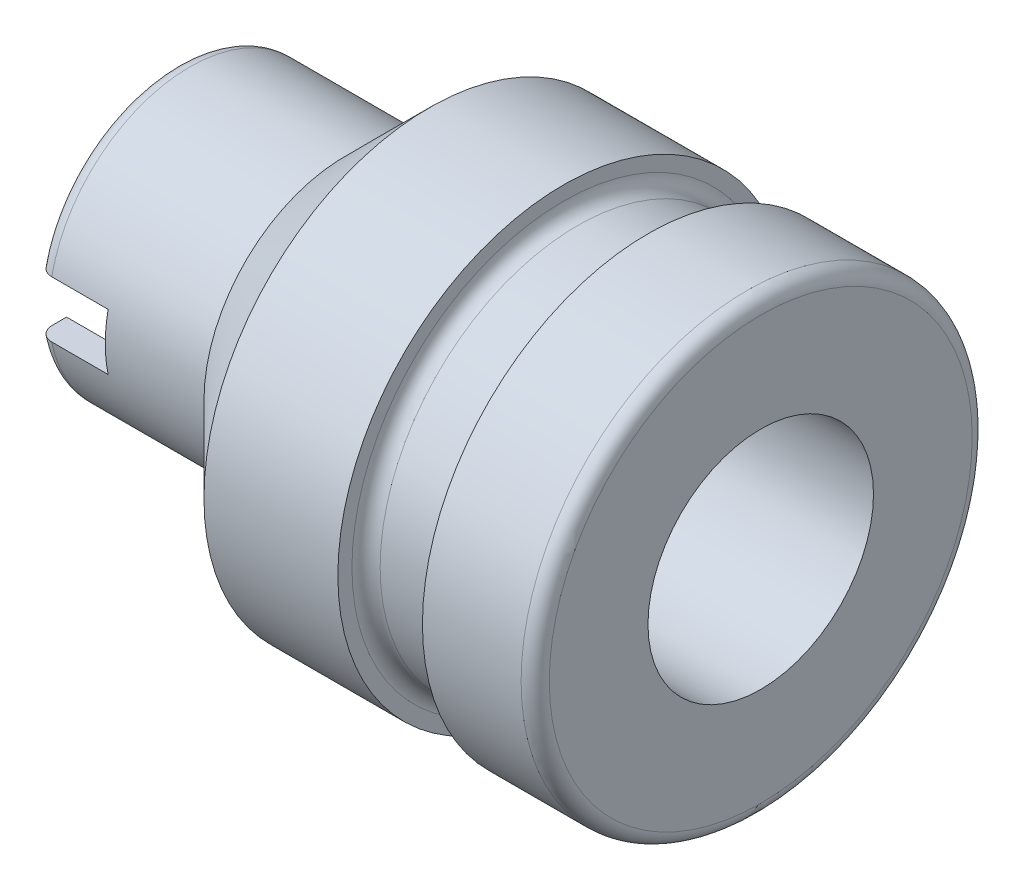
ISO-10303-21;
HEADER;
FILE_DESCRIPTION(('STEP AP214'),'2;1');
FILE_NAME('part.step','',(''),(''),'','','');
FILE_SCHEMA(('AUTOMOTIVE_DESIGN { 1 0 10303 214 1 1 1 1 }'));
ENDSEC;
DATA;
#1=APPLICATION_CONTEXT('core data for automotive mechanical design processes');
#2=APPLICATION_PROTOCOL_DEFINITION('international standard','automotive_design',2000,#1);
#3=PRODUCT_CONTEXT('',#1,'mechanical');
#4=PRODUCT('Part','Part','',(#3));
#5=PRODUCT_RELATED_PRODUCT_CATEGORY('part','',(#4));
#6=PRODUCT_DEFINITION_FORMATION('','',#4);
#7=PRODUCT_DEFINITION_CONTEXT('part definition',#1,'design');
#8=PRODUCT_DEFINITION('design','',#6,#7);
#9=PRODUCT_DEFINITION_SHAPE('','',#8);
#10=(LENGTH_UNIT() NAMED_UNIT(*) SI_UNIT(.MILLI.,.METRE.));
#11=(NAMED_UNIT(*) PLANE_ANGLE_UNIT() SI_UNIT($,.RADIAN.));
#12=(NAMED_UNIT(*) SI_UNIT($,.STERADIAN.) SOLID_ANGLE_UNIT());
#13=UNCERTAINTY_MEASURE_WITH_UNIT(LENGTH_MEASURE(1.E-05),#10,'distance_accuracy_value','');
#14=(GEOMETRIC_REPRESENTATION_CONTEXT(3) GLOBAL_UNCERTAINTY_ASSIGNED_CONTEXT((#13)) GLOBAL_UNIT_ASSIGNED_CONTEXT((#10,
#11,#12)) REPRESENTATION_CONTEXT('',''));
#15=CARTESIAN_POINT('',(0.,0.,0.));
#16=DIRECTION('',(0.,0.,1.));
#17=DIRECTION('',(1.,0.,0.));
#18=AXIS2_PLACEMENT_3D('',#15,#16,#17);
#19=CARTESIAN_POINT('',(0.,0.,0.));
#20=DIRECTION('',(-1.,0.,0.));
#21=DIRECTION('',(0.,0.,1.));
#22=AXIS2_PLACEMENT_3D('',#19,#20,#21);
#23=PLANE('',#22);
#24=DIRECTION('',(0.,0.,1.));
#25=VECTOR('',#24,1.);
#26=CARTESIAN_POINT('',(0.,10.,-16.));
#27=LINE('',#26,#25);
#28=CARTESIAN_POINT('',(0.,10.,7.74596669241483));
#29=VERTEX_POINT('',#28);
#30=CARTESIAN_POINT('',(0.,10.,8.7749643873921));
#31=VERTEX_POINT('',#30);
#32=EDGE_CURVE('E194',#29,#31,#27,.T.);
#33=ORIENTED_EDGE('',*,*,#32,.T.);
#34=CARTESIAN_POINT('',(0.,8.,0.));
#35=DIRECTION('',(-1.,0.,0.));
#36=DIRECTION('',(0.,0.,1.));
#37=AXIS2_PLACEMENT_3D('',#34,#35,#36);
#38=CIRCLE('',#37,8.99999999999998);
#39=CARTESIAN_POINT('',(0.,10.,-8.77496438739202));
#40=VERTEX_POINT('',#39);
#41=EDGE_CURVE('E220',#31,#40,#38,.T.);
#42=ORIENTED_EDGE('',*,*,#41,.T.);
#43=CARTESIAN_POINT('',(0.,10.,-7.74596669241483));
#44=VERTEX_POINT('',#43);
#45=EDGE_CURVE('E193',#40,#44,#27,.T.);
#46=ORIENTED_EDGE('',*,*,#45,.T.);
#47=CARTESIAN_POINT('',(0.,8.,0.));
#48=DIRECTION('',(-1.,0.,0.));
#49=DIRECTION('',(0.,0.,1.));
#50=AXIS2_PLACEMENT_3D('',#47,#48,#49);
#51=CIRCLE('',#50,8.);
#52=EDGE_CURVE('E223',#29,#44,#51,.T.);
#53=ORIENTED_EDGE('',*,*,#52,.F.);
#54=EDGE_LOOP('',(#33,#42,#46,#53));
#55=FACE_BOUND('',#54,.T.);
#56=ADVANCED_FACE('F44',(#55),#23,.T.);
#57=CARTESIAN_POINT('',(1.,8.,0.));
#58=DIRECTION('',(-1.,0.,0.));
#59=DIRECTION('',(0.,0.,1.));
#60=AXIS2_PLACEMENT_3D('',#57,#58,#59);
#61=TOROIDAL_SURFACE('',#60,8.99999999999998,1.);
#62=CARTESIAN_POINT('',(0.511306825927035,10.,-9.6677495790696));
#63=CARTESIAN_POINT('',(0.559308281722965,10.,-9.69520351096408));
#64=CARTESIAN_POINT('',(0.609639032154946,10.,-9.71865802064844));
#65=CARTESIAN_POINT('',(0.713558242155809,10.,-9.75681559968103));
#66=CARTESIAN_POINT('',(0.767149945956613,10.,-9.77150979140529));
#67=CARTESIAN_POINT('',(0.876043559476013,10.,-9.79166035519747));
#68=CARTESIAN_POINT('',(0.931345300899028,10.,-9.79711763340043));
#69=CARTESIAN_POINT('',(1.04206355524924,10.,-9.79861988345027));
#70=CARTESIAN_POINT('',(1.09748004028236,10.,-9.7946669235582));
#71=CARTESIAN_POINT('',(1.20660988208594,10.,-9.77751812422735));
#72=CARTESIAN_POINT('',(1.26032970143437,10.,-9.76436334861136));
#73=CARTESIAN_POINT('',(1.36481599217086,10.,-9.72926499149187));
#74=CARTESIAN_POINT('',(1.41558235227585,10.,-9.70732107906873));
#75=CARTESIAN_POINT('',(1.51301248392595,10.,-9.65518458376579));
#76=CARTESIAN_POINT('',(1.5596543139653,10.,-9.62495102864483));
#77=CARTESIAN_POINT('',(1.647298612418,10.,-9.5571938737038));
#78=CARTESIAN_POINT('',(1.68830072482487,10.,-9.51966981403191));
#79=CARTESIAN_POINT('',(1.76419505830093,10.,-9.43779402545148));
#80=CARTESIAN_POINT('',(1.79898312438137,10.,-9.39334578929934));
#81=CARTESIAN_POINT('',(1.86078526900064,10.,-9.29934095322765));
#82=CARTESIAN_POINT('',(1.88779856031153,10.,-9.24978383670244));
#83=CARTESIAN_POINT('',(1.93389245120233,10.,-9.14584851749056));
#84=CARTESIAN_POINT('',(1.95279295699506,10.,-9.09139044671483));
#85=CARTESIAN_POINT('',(1.98138125003641,10.,-8.98010780940885));
#86=CARTESIAN_POINT('',(1.99106799193015,10.,-8.9232829751188));
#87=CARTESIAN_POINT('',(2.00112427890071,10.,-8.80768146328481));
#88=CARTESIAN_POINT('',(2.00130601462751,10.,-8.74888840256496));
#89=CARTESIAN_POINT('',(1.9919017520578,10.,-8.63208632529093));
#90=CARTESIAN_POINT('',(1.98231495867919,10.,-8.57407737294647));
#91=CARTESIAN_POINT('',(1.95348329284294,10.,-8.45989655601053));
#92=CARTESIAN_POINT('',(1.93414395709675,10.,-8.40374849719579));
#93=CARTESIAN_POINT('',(1.8862524674463,10.,-8.29552412270311));
#94=CARTESIAN_POINT('',(1.85770032889892,10.,-8.24344780023816));
#95=CARTESIAN_POINT('',(1.79234125019335,10.,-8.14526750270985));
#96=CARTESIAN_POINT('',(1.75559179207176,10.,-8.09912530594951));
#97=CARTESIAN_POINT('',(1.67469797107571,10.,-8.01385024714823));
#98=CARTESIAN_POINT('',(1.63055451541159,10.,-7.97471652641611));
#99=CARTESIAN_POINT('',(1.53721783151604,10.,-7.90558984461912));
#100=CARTESIAN_POINT('',(1.48816814766731,10.,-7.87540317887255));
#101=CARTESIAN_POINT('',(1.38557805500345,10.,-7.82398855871157));
#102=CARTESIAN_POINT('',(1.33203850957662,10.,-7.80275888660533));
#103=CARTESIAN_POINT('',(1.22370997690863,10.,-7.77050867101741));
#104=CARTESIAN_POINT('',(1.16900603361279,10.,-7.75920221435131));
#105=CARTESIAN_POINT('',(1.05847182518937,10.,-7.74613510599163));
#106=CARTESIAN_POINT('',(1.00264171380159,10.,-7.74437316005553));
#107=CARTESIAN_POINT('',(0.892582708877808,10.,-7.75039635440434));
#108=CARTESIAN_POINT('',(0.838343678634541,10.,-7.75799839748392));
#109=CARTESIAN_POINT('',(0.731908480522575,10.,-7.78217880416063));
#110=CARTESIAN_POINT('',(0.679712293696711,10.,-7.79875708443894));
#111=CARTESIAN_POINT('',(0.578658081208827,10.,-7.84039550056985));
#112=CARTESIAN_POINT('',(0.529809656562754,10.,-7.86547889710702));
#113=CARTESIAN_POINT('',(0.43689225974382,10.,-7.92331749551591));
#114=CARTESIAN_POINT('',(0.392823751135206,10.,-7.95607344051264));
#115=CARTESIAN_POINT('',(0.309637769043108,10.,-8.02908979521609));
#116=CARTESIAN_POINT('',(0.270654071066901,10.,-8.06950253140811));
#117=CARTESIAN_POINT('',(0.199789029681809,10.,-8.15613564920241));
#118=CARTESIAN_POINT('',(0.167908744225208,10.,-8.20235689429834));
#119=CARTESIAN_POINT('',(0.11118055267698,10.,-8.3007507838291));
#120=CARTESIAN_POINT('',(0.0865663966446748,10.,-8.35305824482765));
#121=CARTESIAN_POINT('',(0.0462562889607229,10.,-8.46100433264482));
#122=CARTESIAN_POINT('',(0.0305614855014643,10.,-8.51664338732247));
#123=CARTESIAN_POINT('',(0.00823822667101209,10.,-8.63095929611147));
#124=CARTESIAN_POINT('',(0.00181209474607875,10.,-8.68967575315516));
#125=CARTESIAN_POINT('',(-0.001147154551948,10.,-8.80735800605802));
#126=CARTESIAN_POINT('',(0.00231987019037505,10.,-8.86632380548684));
#127=CARTESIAN_POINT('',(0.0191336971782254,10.,-8.98312733812228));
#128=CARTESIAN_POINT('',(0.0325285171266589,10.,-9.04095818168231));
#129=CARTESIAN_POINT('',(0.068952109280189,10.,-9.15352293406955));
#130=CARTESIAN_POINT('',(0.091982863025496,10.,-9.2082562032797));
#131=CARTESIAN_POINT('',(0.146792032565864,10.,-9.31239064575795));
#132=CARTESIAN_POINT('',(0.178472817770748,10.,-9.36184323216501));
#133=CARTESIAN_POINT('',(0.249831530740876,10.,-9.45453280413945));
#134=CARTESIAN_POINT('',(0.289498801103796,10.,-9.4977779427507));
#135=CARTESIAN_POINT('',(0.35984513733962,10.,-9.56220360357953));
#136=CARTESIAN_POINT('',(0.388477869102997,10.,-9.5856561085426));
#137=CARTESIAN_POINT('',(0.448162302179852,10.,-9.62925148252653));
#138=CARTESIAN_POINT('',(0.479213966106138,10.,-9.64939440268562));
#139=CARTESIAN_POINT('',(0.511306825927035,10.,-9.6677495790696));
#140=B_SPLINE_CURVE_WITH_KNOTS('',3,(#62,#63,#64,#65,#66,#67,#68,#69,#70,#71,#72,#73,#74,#75,
#76,#77,#78,#79,#80,#81,#82,#83,#84,#85,#86,#87,#88,#89,#90,#91,#92,#93,#94,#95,#96,#97,#98,#99,
#100,#101,#102,#103,#104,#105,#106,#107,#108,#109,#110,#111,#112,#113,#114,#115,#116,#117,#118,
#119,#120,#121,#122,#123,#124,#125,#126,#127,#128,#129,#130,#131,#132,#133,#134,#135,#136,#137,
#138,#139),.UNSPECIFIED.,.T.,.F.,(4,2,2,2,2,2,2,2,2,2,2,2,2,2,2,2,2,2,2,2,2,2,2,2,2,2,2,2,2,2,2,
2,2,2,2,2,2,2,4),(0.,0.165760656846688,0.331689009703769,0.497601084156693,0.66347669642919,
0.828616759413993,0.993763040669096,1.15974076125184,1.32572895435387,1.49428098685655,
1.66285007994709,1.8349887499326,2.0071469477183,2.18270555882353,2.35827846017236,
2.53558560043269,2.71289244514009,2.88899300563287,3.06507197518268,3.23700082338466,
3.40889668561266,3.57565978746695,3.74240027555845,3.90593155970491,4.06946132595477,
4.23344198705861,4.39743853708843,4.56512660663086,4.7328396342577,4.9054729168679,
5.0781284176095,5.25449852909511,5.43087117415406,5.60810249270579,5.78537027515778,
5.96071456378588,6.13582640039848,6.24665253354264,6.35747695408974),.UNSPECIFIED.);
#141=CARTESIAN_POINT('',(1.,10.,-9.79795897113269));
#142=VERTEX_POINT('',#141);
#143=EDGE_CURVE('E156',#40,#142,#140,.T.);
#144=ORIENTED_EDGE('',*,*,#143,.F.);
#145=ORIENTED_EDGE('',*,*,#41,.F.);
#146=CARTESIAN_POINT('',(0.530086633266854,10.,7.8670423739127));
#147=CARTESIAN_POINT('',(0.578141397714327,10.,7.84064914283677));
#148=CARTESIAN_POINT('',(0.628419871150143,10.,7.81823476131326));
#149=CARTESIAN_POINT('',(0.732054975608554,10.,7.78212334392136));
#150=CARTESIAN_POINT('',(0.785414272238746,10.,7.76843398426953));
#151=CARTESIAN_POINT('',(0.893694754150047,10.,7.7502583049771));
#152=CARTESIAN_POINT('',(0.94861621718662,10.,7.74577363244534));
#153=CARTESIAN_POINT('',(1.05841316345902,10.,7.74617251060403));
#154=CARTESIAN_POINT('',(1.1132886538094,10.,7.75105414228967));
#155=CARTESIAN_POINT('',(1.22101648805253,10.,7.76993821482575));
#156=CARTESIAN_POINT('',(1.27388095611584,10.,7.78387168868395));
#157=CARTESIAN_POINT('',(1.37655874242189,10.,7.82032521094701));
#158=CARTESIAN_POINT('',(1.42637187394239,10.,7.8428457842193));
#159=CARTESIAN_POINT('',(1.52213173794623,10.,7.89603321356496));
#160=CARTESIAN_POINT('',(1.56803166365623,10.,7.92678424161405));
#161=CARTESIAN_POINT('',(1.65419034084942,10.,7.9953682486375));
#162=CARTESIAN_POINT('',(1.69444840750263,10.,8.03320208605009));
#163=CARTESIAN_POINT('',(1.76933370530235,10.,8.11594516892443));
#164=CARTESIAN_POINT('',(1.8037821363678,10.,8.16101619860671));
#165=CARTESIAN_POINT('',(1.8648692450916,10.,8.25617083413549));
#166=CARTESIAN_POINT('',(1.89150677818158,10.,8.30625517316537));
#167=CARTESIAN_POINT('',(1.93697477776608,10.,8.41152787043869));
#168=CARTESIAN_POINT('',(1.9555650521892,10.,8.46682005042279));
#169=CARTESIAN_POINT('',(1.98336758010917,10.,8.57971552998892));
#170=CARTESIAN_POINT('',(1.99257883459075,10.,8.63731907508913));
#171=CARTESIAN_POINT('',(2.00145172674255,10.,8.75420255934511));
#172=CARTESIAN_POINT('',(2.00095588058722,10.,8.81349453153748));
#173=CARTESIAN_POINT('',(1.99000786091946,10.,8.93115517583231));
#174=CARTESIAN_POINT('',(1.97955550413699,10.,8.98952383091912));
#175=CARTESIAN_POINT('',(1.94894306490324,10.,9.10358714712749));
#176=CARTESIAN_POINT('',(1.92879463966272,10.,9.15928493113948));
#177=CARTESIAN_POINT('',(1.87928764906859,10.,9.26642836714244));
#178=CARTESIAN_POINT('',(1.84992973339864,10.,9.31787431875565));
#179=CARTESIAN_POINT('',(1.78330190216955,10.,9.41417425155647));
#180=CARTESIAN_POINT('',(1.74616272288383,10.,9.45911864051572));
#181=CARTESIAN_POINT('',(1.66471340194489,10.,9.54195979436287));
#182=CARTESIAN_POINT('',(1.62040412592035,10.,9.57985740880559));
#183=CARTESIAN_POINT('',(1.52691131817347,10.,9.64664863756471));
#184=CARTESIAN_POINT('',(1.47785526132285,10.,9.67572069984084));
#185=CARTESIAN_POINT('',(1.37548685852437,10.,9.72502935448071));
#186=CARTESIAN_POINT('',(1.32217501009044,10.,9.74526697783106));
#187=CARTESIAN_POINT('',(1.21391011756111,10.,9.77595055141352));
#188=CARTESIAN_POINT('',(1.15900809567203,10.,9.78657669499911));
#189=CARTESIAN_POINT('',(1.04819822807474,10.,9.79835661860274));
#190=CARTESIAN_POINT('',(0.992290455428851,10.,9.79951108392428));
#191=CARTESIAN_POINT('',(0.881654127451369,10.,9.79234847781777));
#192=CARTESIAN_POINT('',(0.826919366226506,10.,9.78412675678912));
#193=CARTESIAN_POINT('',(0.719604454653113,10.,9.75862572790174));
#194=CARTESIAN_POINT('',(0.667024283713556,10.,9.74134650662567));
#195=CARTESIAN_POINT('',(0.565390440348432,10.,9.69822660717811));
#196=CARTESIAN_POINT('',(0.516343373928049,10.,9.67237037327907));
#197=CARTESIAN_POINT('',(0.423212995336157,10.,9.61289096461068));
#198=CARTESIAN_POINT('',(0.379129927662664,10.,9.57926740751637));
#199=CARTESIAN_POINT('',(0.296548199057912,10.,9.50476302258947));
#200=CARTESIAN_POINT('',(0.258129456500358,10.,9.46379365494053));
#201=CARTESIAN_POINT('',(0.188551954038964,10.,9.37609769672073));
#202=CARTESIAN_POINT('',(0.157393896303961,10.,9.32937054999207));
#203=CARTESIAN_POINT('',(0.102544847496919,10.,9.23047974526343));
#204=CARTESIAN_POINT('',(0.0790177674306911,10.,9.17822518894706));
#205=CARTESIAN_POINT('',(0.0408664514457591,10.,9.07056209938669));
#206=CARTESIAN_POINT('',(0.026243238739463,10.,9.01515320445294));
#207=CARTESIAN_POINT('',(0.00601242351154127,10.,8.90151246286388));
#208=CARTESIAN_POINT('',(0.000600274872774322,10.,8.8432457862255));
#209=CARTESIAN_POINT('',(-0.000505796595671923,10.,8.72662072581589));
#210=CARTESIAN_POINT('',(0.00380084075076319,10.,8.66826233695224));
#211=CARTESIAN_POINT('',(0.0221249794561776,10.,8.55229379625042));
#212=CARTESIAN_POINT('',(0.0362704171598719,10.,8.49470380971241));
#213=CARTESIAN_POINT('',(0.0740488816321859,10.,8.38270291383713));
#214=CARTESIAN_POINT('',(0.0976844683595091,10.,8.3282928668258));
#215=CARTESIAN_POINT('',(0.153795894139131,10.,8.22434078489802));
#216=CARTESIAN_POINT('',(0.186259004324004,10.,8.17479187937067));
#217=CARTESIAN_POINT('',(0.259176927714039,10.,8.08203325396201));
#218=CARTESIAN_POINT('',(0.299621370850104,10.,8.03881543379349));
#219=CARTESIAN_POINT('',(0.371936794602742,10.,7.9739318252388));
#220=CARTESIAN_POINT('',(0.401830277842509,10.,7.95002752103271));
#221=CARTESIAN_POINT('',(0.464151019596761,10.,7.90578479045156));
#222=CARTESIAN_POINT('',(0.496578217983059,10.,7.88544627949296));
#223=CARTESIAN_POINT('',(0.530086633266854,10.,7.8670423739127));
#224=B_SPLINE_CURVE_WITH_KNOTS('',3,(#146,#147,#148,#149,#150,#151,#152,#153,#154,#155,#156,
#157,#158,#159,#160,#161,#162,#163,#164,#165,#166,#167,#168,#169,#170,#171,#172,#173,#174,#175,
#176,#177,#178,#179,#180,#181,#182,#183,#184,#185,#186,#187,#188,#189,#190,#191,#192,#193,#194,
#195,#196,#197,#198,#199,#200,#201,#202,#203,#204,#205,#206,#207,#208,#209,#210,#211,#212,#213,
#214,#215,#216,#217,#218,#219,#220,#221,#222,#223),.UNSPECIFIED.,.T.,.F.,(4,2,2,2,2,2,2,2,2,2,2,
2,2,2,2,2,2,2,2,2,2,2,2,2,2,2,2,2,2,2,2,2,2,2,2,2,2,2,4),(0.,0.164341324993714,
0.328827037538444,0.493342180986613,0.657823621532061,0.821066328878155,0.984319015672965,
1.14930967077576,1.31432033574771,1.48373163535811,1.6531677472279,1.827361011495,
2.00157282818377,2.17861329102043,2.35565701271359,2.53248841130041,2.70930733811718,
2.88336459438589,3.05740085279306,3.22763906699898,3.3978574089444,3.56481409859054,
3.73175870832779,3.89702061163649,4.06228093519885,4.22784263754271,4.39341249093985,
4.56113157984433,4.72886688185976,4.8999974046941,5.07114758975335,5.24588619185384,
5.42063486588012,5.59769938739947,5.77481170402832,5.95166997514037,6.12829995124597,
6.24289728777437,6.35749190559209),.UNSPECIFIED.);
#225=CARTESIAN_POINT('',(1.,10.,9.79795897113269));
#226=VERTEX_POINT('',#225);
#227=EDGE_CURVE('E150',#226,#31,#224,.T.);
#228=ORIENTED_EDGE('',*,*,#227,.F.);
#229=CARTESIAN_POINT('',(1.,8.,0.));
#230=DIRECTION('',(-1.,0.,0.));
#231=DIRECTION('',(0.,0.,1.));
#232=AXIS2_PLACEMENT_3D('',#229,#230,#231);
#233=CIRCLE('',#232,9.99999999999998);
#234=EDGE_CURVE('E217',#226,#142,#233,.T.);
#235=ORIENTED_EDGE('',*,*,#234,.T.);
#236=EDGE_LOOP('',(#144,#145,#228,#235));
#237=FACE_BOUND('',#236,.T.);
#238=ADVANCED_FACE('F248',(#237),#61,.T.);
#239=CARTESIAN_POINT('',(-18.7543710445799,8.,0.));
#240=DIRECTION('',(-1.,0.,0.));
#241=DIRECTION('',(0.,0.,1.));
#242=AXIS2_PLACEMENT_3D('',#239,#240,#241);
#243=CYLINDRICAL_SURFACE('',#242,8.);
#244=DIRECTION('',(-1.,0.,0.));
#245=VECTOR('',#244,1.);
#246=CARTESIAN_POINT('',(-18.7543710445799,10.,7.74596669241483));
#247=LINE('',#246,#245);
#248=CARTESIAN_POINT('',(5.,10.,7.74596669241483));
#249=VERTEX_POINT('',#248);
#250=EDGE_CURVE('E239',#29,#249,#247,.F.);
#251=ORIENTED_EDGE('',*,*,#250,.F.);
#252=ORIENTED_EDGE('',*,*,#52,.T.);
#253=DIRECTION('',(-1.,0.,0.));
#254=VECTOR('',#253,1.);
#255=CARTESIAN_POINT('',(-18.7543710445799,10.,-7.74596669241483));
#256=LINE('',#255,#254);
#257=CARTESIAN_POINT('',(5.,10.,-7.74596669241483));
#258=VERTEX_POINT('',#257);
#259=EDGE_CURVE('E145',#258,#44,#256,.T.);
#260=ORIENTED_EDGE('',*,*,#259,.F.);
#261=CARTESIAN_POINT('',(5.,8.,0.));
#262=DIRECTION('',(1.,0.,0.));
#263=DIRECTION('',(0.,0.,-1.));
#264=AXIS2_PLACEMENT_3D('',#261,#262,#263);
#265=CIRCLE('',#264,8.);
#266=CARTESIAN_POINT('',(5.,6.,-7.74596669241483));
#267=VERTEX_POINT('',#266);
#268=EDGE_CURVE('E135',#267,#258,#265,.T.);
#269=ORIENTED_EDGE('',*,*,#268,.F.);
#270=DIRECTION('',(-1.,0.,0.));
#271=VECTOR('',#270,1.);
#272=CARTESIAN_POINT('',(-18.7543710445799,6.,-7.74596669241483));
#273=LINE('',#272,#271);
#274=CARTESIAN_POINT('',(0.,6.,-7.74596669241483));
#275=VERTEX_POINT('',#274);
#276=EDGE_CURVE('E116',#275,#267,#273,.F.);
#277=ORIENTED_EDGE('',*,*,#276,.F.);
#278=CARTESIAN_POINT('',(0.,6.,7.74596669241483));
#279=VERTEX_POINT('',#278);
#280=EDGE_CURVE('E219',#275,#279,#51,.T.);
#281=ORIENTED_EDGE('',*,*,#280,.T.);
#282=DIRECTION('',(-1.,0.,0.));
#283=VECTOR('',#282,1.);
#284=CARTESIAN_POINT('',(-18.7543710445799,6.,7.74596669241483));
#285=LINE('',#284,#283);
#286=CARTESIAN_POINT('',(5.,6.,7.74596669241483));
#287=VERTEX_POINT('',#286);
#288=EDGE_CURVE('E130',#287,#279,#285,.T.);
#289=ORIENTED_EDGE('',*,*,#288,.F.);
#290=EDGE_CURVE('E144',#249,#287,#265,.T.);
#291=ORIENTED_EDGE('',*,*,#290,.F.);
#292=EDGE_LOOP('',(#251,#252,#260,#269,#277,#281,#289,#291));
#293=FACE_BOUND('',#292,.T.);
#294=CARTESIAN_POINT('',(41.5,8.,0.));
#295=DIRECTION('',(-1.,0.,0.));
#296=DIRECTION('',(0.,0.,1.));
#297=AXIS2_PLACEMENT_3D('',#294,#295,#296);
#298=CIRCLE('',#297,7.99999999999999);
#299=CARTESIAN_POINT('',(41.5,8.,7.99999999999999));
#300=VERTEX_POINT('',#299);
#301=EDGE_CURVE('E246',#300,#300,#298,.T.);
#302=ORIENTED_EDGE('',*,*,#301,.F.);
#303=EDGE_LOOP('',(#302));
#304=FACE_BOUND('',#303,.T.);
#305=ADVANCED_FACE('F50',(#293,#304),#243,.F.);
#306=DIRECTION('',(0.,0.,1.));
#307=VECTOR('',#306,1.);
#308=CARTESIAN_POINT('',(0.,6.,-16.));
#309=LINE('',#308,#307);
#310=CARTESIAN_POINT('',(0.,6.,-8.77496438739146));
#311=VERTEX_POINT('',#310);
#312=EDGE_CURVE('E125',#311,#275,#309,.T.);
#313=ORIENTED_EDGE('',*,*,#312,.F.);
#314=CARTESIAN_POINT('',(0.,6.,8.77496438739227));
#315=VERTEX_POINT('',#314);
#316=EDGE_CURVE('E213',#311,#315,#38,.T.);
#317=ORIENTED_EDGE('',*,*,#316,.T.);
#318=EDGE_CURVE('E204',#279,#315,#309,.T.);
#319=ORIENTED_EDGE('',*,*,#318,.F.);
#320=ORIENTED_EDGE('',*,*,#280,.F.);
#321=EDGE_LOOP('',(#313,#317,#319,#320));
#322=FACE_BOUND('',#321,.T.);
#323=ADVANCED_FACE('F216',(#322),#23,.T.);
#324=CARTESIAN_POINT('',(0.511306825927035,6.,-9.6677495790696));
#325=CARTESIAN_POINT('',(0.462127792878772,6.,-9.63961614014446));
#326=CARTESIAN_POINT('',(0.415321432721198,6.,-9.60724164376228));
#327=CARTESIAN_POINT('',(0.327807674940792,6.,-9.53502366722364));
#328=CARTESIAN_POINT('',(0.287109053947641,6.,-9.49516962067705));
#329=CARTESIAN_POINT('',(0.212996868443189,6.,-9.40927866329832));
#330=CARTESIAN_POINT('',(0.179573316452268,6.,-9.36325037090132));
#331=CARTESIAN_POINT('',(0.120796696181657,6.,-9.26632548183998));
#332=CARTESIAN_POINT('',(0.0954416705950956,6.,-9.21543006976995));
#333=CARTESIAN_POINT('',(0.05305026963304,6.,-9.10933538170457));
#334=CARTESIAN_POINT('',(0.0361541675774601,6.,-9.05408007300957));
#335=CARTESIAN_POINT('',(0.0116835589855953,6.,-8.94153981509048));
#336=CARTESIAN_POINT('',(0.00411048112851551,6.,-8.88425455617609));
#337=CARTESIAN_POINT('',(-0.00161449656823779,6.,-8.76811550635739));
#338=CARTESIAN_POINT('',(0.000416367341279644,6.,-8.7092526583363));
#339=CARTESIAN_POINT('',(0.0142429607025673,6.,-8.59268248788178));
#340=CARTESIAN_POINT('',(0.0260394125136054,6.,-8.53497525125219));
#341=CARTESIAN_POINT('',(0.0592295532006887,6.,-8.42186663703923));
#342=CARTESIAN_POINT('',(0.0807017165191936,6.,-8.36648824519507));
#343=CARTESIAN_POINT('',(0.132717456638743,6.,-8.26016420202981));
#344=CARTESIAN_POINT('',(0.163260879747507,6.,-8.20921847562597));
#345=CARTESIAN_POINT('',(0.232319712500392,6.,-8.11373419885014));
#346=CARTESIAN_POINT('',(0.270761984519968,6.,-8.06914281018449));
#347=CARTESIAN_POINT('',(0.35475961241516,6.,-7.9872504066813));
#348=CARTESIAN_POINT('',(0.400314015263732,6.,-7.94994841656858));
#349=CARTESIAN_POINT('',(0.49603998492741,6.,-7.88472033956897));
#350=CARTESIAN_POINT('',(0.546067638456784,6.,-7.85658315502762));
#351=CARTESIAN_POINT('',(0.650242201905039,6.,-7.80940325123956));
#352=CARTESIAN_POINT('',(0.704388317457524,6.,-7.79035878332612));
#353=CARTESIAN_POINT('',(0.81354111836697,6.,-7.76246756444927));
#354=CARTESIAN_POINT('',(0.868475209312162,6.,-7.75333635979499));
#355=CARTESIAN_POINT('',(0.97909332477837,6.,-7.74460503194061));
#356=CARTESIAN_POINT('',(1.03477725649985,6.,-7.74500373996807));
#357=CARTESIAN_POINT('',(1.14430583108474,6.,-7.75522657668602));
#358=CARTESIAN_POINT('',(1.19816564263771,6.,-7.76488932614733));
#359=CARTESIAN_POINT('',(1.30351120575465,6.,-7.79307437632797));
#360=CARTESIAN_POINT('',(1.35499694668112,6.,-7.8115967167403));
#361=CARTESIAN_POINT('',(1.45446136037515,6.,-7.85701332402369));
#362=CARTESIAN_POINT('',(1.50241974199559,6.,-7.8839519606661));
#363=CARTESIAN_POINT('',(1.59327424205895,6.,-7.94531836244351));
#364=CARTESIAN_POINT('',(1.63616981903902,6.,-7.97974692750276));
#365=CARTESIAN_POINT('',(1.71679853240975,6.,-8.05598011482791));
#366=CARTESIAN_POINT('',(1.75438273298845,6.,-8.09794219253199));
#367=CARTESIAN_POINT('',(1.82221388314016,6.,-8.18742637731591));
#368=CARTESIAN_POINT('',(1.85245974598291,6.,-8.23494930635633));
#369=CARTESIAN_POINT('',(1.90566745527039,6.,-8.33569399048775));
#370=CARTESIAN_POINT('',(1.92839144874395,6.,-8.38904142784494));
#371=CARTESIAN_POINT('',(1.96476097282934,6.,-8.49874705230807));
#372=CARTESIAN_POINT('',(1.97840540022242,6.,-8.55510560438308));
#373=CARTESIAN_POINT('',(1.99645269595044,6.,-8.67043761172828));
#374=CARTESIAN_POINT('',(2.00066621894879,6.,-8.72944078635048));
#375=CARTESIAN_POINT('',(1.99916261837003,6.,-8.84732326181367));
#376=CARTESIAN_POINT('',(1.9934450951045,6.,-8.9062025575735));
#377=CARTESIAN_POINT('',(1.97215664019017,6.,-9.02233734661196));
#378=CARTESIAN_POINT('',(1.95655657656459,6.,-9.07958751434796));
#379=CARTESIAN_POINT('',(1.9158429235496,6.,-9.19060252497679));
#380=CARTESIAN_POINT('',(1.89072980594297,6.,-9.24436754055462));
#381=CARTESIAN_POINT('',(1.8320123031712,6.,-9.34612633467259));
#382=CARTESIAN_POINT('',(1.79852090549833,6.,-9.39418526504363));
#383=CARTESIAN_POINT('',(1.72378285853897,6.,-9.4838415356261));
#384=CARTESIAN_POINT('',(1.68253707794454,6.,-9.52543959866999));
#385=CARTESIAN_POINT('',(1.59439479967278,6.,-9.60004783335381));
#386=CARTESIAN_POINT('',(1.54763644474854,6.,-9.633221197224));
#387=CARTESIAN_POINT('',(1.44912221996927,6.,-9.69105176991122));
#388=CARTESIAN_POINT('',(1.39736716585799,6.,-9.7157103658215));
#389=CARTESIAN_POINT('',(1.29147850342786,6.,-9.75529780839208));
#390=CARTESIAN_POINT('',(1.23741588921197,6.,-9.77041668772133));
#391=CARTESIAN_POINT('',(1.12749141216315,6.,-9.79123670479128));
#392=CARTESIAN_POINT('',(1.07162923502451,6.,-9.79693618817954));
#393=CARTESIAN_POINT('',(0.960438790024008,6.,-9.798719451814));
#394=CARTESIAN_POINT('',(0.905112274476687,6.,-9.79491913855203));
#395=CARTESIAN_POINT('',(0.795937463990675,6.,-9.7780659133441));
#396=CARTESIAN_POINT('',(0.742087362546607,6.,-9.76502488581324));
#397=CARTESIAN_POINT('',(0.658775688732057,6.,-9.73727365800327));
#398=CARTESIAN_POINT('',(0.62833254518202,6.,-9.7254183911905));
#399=CARTESIAN_POINT('',(0.568765995941057,6.,-9.69876122999197));
#400=CARTESIAN_POINT('',(0.539642573272034,6.,-9.68395937352706));
#401=CARTESIAN_POINT('',(0.511306825927035,6.,-9.6677495790696));
#402=B_SPLINE_CURVE_WITH_KNOTS('',3,(#324,#325,#326,#327,#328,#329,#330,#331,#332,#333,#334,
#335,#336,#337,#338,#339,#340,#341,#342,#343,#344,#345,#346,#347,#348,#349,#350,#351,#352,#353,
#354,#355,#356,#357,#358,#359,#360,#361,#362,#363,#364,#365,#366,#367,#368,#369,#370,#371,#372,
#373,#374,#375,#376,#377,#378,#379,#380,#381,#382,#383,#384,#385,#386,#387,#388,#389,#390,#391,
#392,#393,#394,#395,#396,#397,#398,#399,#400,#401),.UNSPECIFIED.,.T.,.F.,(4,2,2,2,2,2,2,2,2,2,2,
2,2,2,2,2,2,2,2,2,2,2,2,2,2,2,2,2,2,2,2,2,2,2,2,2,2,2,4),(0.,0.169850150266518,
0.339942079778361,0.50979900715325,0.679614698247264,0.852160160522137,1.02473206072483,
1.20060108857805,1.37648312660291,1.55381806451728,1.73114999805774,1.9069085174148,
2.08264350527523,2.25398479513653,2.42529312019405,2.59154417777022,2.75777484600336,
2.92116142093442,3.08454872788159,3.24881235821947,3.41309354053031,3.58132496241899,
3.74958128241785,3.92273898784218,4.09591772906961,4.27254334638773,4.44917607240782,
4.62633191879003,4.80347898059724,4.97835497749308,5.15321139540125,5.32436534661133,
5.49549140291978,5.66309100644069,5.83072004277876,5.99631385313887,6.16169508014642,
6.25955981194753,6.35742328436958),.UNSPECIFIED.);
#403=CARTESIAN_POINT('',(1.,6.,-9.79795897113269));
#404=VERTEX_POINT('',#403);
#405=EDGE_CURVE('E185',#404,#311,#402,.T.);
#406=ORIENTED_EDGE('',*,*,#405,.F.);
#407=CARTESIAN_POINT('',(1.,6.,9.79795897113269));
#408=VERTEX_POINT('',#407);
#409=EDGE_CURVE('E214',#404,#408,#233,.T.);
#410=ORIENTED_EDGE('',*,*,#409,.T.);
#411=CARTESIAN_POINT('',(0.530086633266854,6.,7.8670423739127));
#412=CARTESIAN_POINT('',(0.480157368302665,6.,7.89447106323999));
#413=CARTESIAN_POINT('',(0.432555263224318,6.,7.92623753753401));
#414=CARTESIAN_POINT('',(0.343366232469098,6.,7.99739457998698));
#415=CARTESIAN_POINT('',(0.301788803444568,6.,8.03679696091914));
#416=CARTESIAN_POINT('',(0.225848412935354,6.,8.12190594718989));
#417=CARTESIAN_POINT('',(0.191473153685613,6.,8.16760158187225));
#418=CARTESIAN_POINT('',(0.130706912853064,6.,8.26399799776451));
#419=CARTESIAN_POINT('',(0.10431388227869,6.,8.31469749007377));
#420=CARTESIAN_POINT('',(0.059659609792196,6.,8.42081562511446));
#421=CARTESIAN_POINT('',(0.0415804860343073,6.,8.47631093054857));
#422=CARTESIAN_POINT('',(0.0148295055883365,6.,8.58952919615366));
#423=CARTESIAN_POINT('',(0.00615907485437737,6.,8.64725249262003));
#424=CARTESIAN_POINT('',(-0.00160282206247777,6.,8.76426286477589));
#425=CARTESIAN_POINT('',(-0.000540352973194271,6.,8.82356022684946));
#426=CARTESIAN_POINT('',(0.0115389002273405,6.,8.94113537889348));
#427=CARTESIAN_POINT('',(0.0225558298288257,6.,8.99941315394937));
#428=CARTESIAN_POINT('',(0.0542721639085431,6.,9.1131704915499));
#429=CARTESIAN_POINT('',(0.0749552215222792,6.,9.16865460378348));
#430=CARTESIAN_POINT('',(0.125490039224446,6.,9.27528071806156));
#431=CARTESIAN_POINT('',(0.155341107326976,6.,9.32642304744473));
#432=CARTESIAN_POINT('',(0.222880835965292,6.,9.4220234591088));
#433=CARTESIAN_POINT('',(0.260437146323016,6.,9.46657499855229));
#434=CARTESIAN_POINT('',(0.342647390407683,6.,9.5485642723794));
#435=CARTESIAN_POINT('',(0.387300473582023,6.,9.58600285807591));
#436=CARTESIAN_POINT('',(0.481387268327656,6.,9.65183275755295));
#437=CARTESIAN_POINT('',(0.530695109231385,6.,9.68040398537549));
#438=CARTESIAN_POINT('',(0.633476804445531,6.,9.72867699847136));
#439=CARTESIAN_POINT('',(0.686950172718174,6.,9.74837981670635));
#440=CARTESIAN_POINT('',(0.795450808649531,6.,9.77799054097276));
#441=CARTESIAN_POINT('',(0.850429334925891,6.,9.7880772190809));
#442=CARTESIAN_POINT('',(0.961299484543756,6.,9.7987762735279));
#443=CARTESIAN_POINT('',(1.01719104331089,6.,9.79938931701191));
#444=CARTESIAN_POINT('',(1.12772227725119,6.,9.7911633925841));
#445=CARTESIAN_POINT('',(1.18236884704737,6.,9.78241663757013));
#446=CARTESIAN_POINT('',(1.28942166501776,6.,9.75589098594791));
#447=CARTESIAN_POINT('',(1.34182793154063,6.,9.73811216333));
#448=CARTESIAN_POINT('',(1.44305235572078,6.,9.69402478522741));
#449=CARTESIAN_POINT('',(1.49186249169897,6.,9.66769782895967));
#450=CARTESIAN_POINT('',(1.58444600478883,6.,9.60732483594793));
#451=CARTESIAN_POINT('',(1.62821912056487,6.,9.57327839896623));
#452=CARTESIAN_POINT('',(1.7101250059956,6.,9.49797173121638));
#453=CARTESIAN_POINT('',(1.74817531823684,6.,9.45662185977551));
#454=CARTESIAN_POINT('',(1.8169593963883,6.,9.36823139184223));
#455=CARTESIAN_POINT('',(1.84769246234981,6.,9.32119025158646));
#456=CARTESIAN_POINT('',(1.90164130914549,6.,9.2217334542379));
#457=CARTESIAN_POINT('',(1.92469125491635,6.,9.16922785481964));
#458=CARTESIAN_POINT('',(1.96185270206181,6.,9.06114425258457));
#459=CARTESIAN_POINT('',(1.97596318551351,6.,9.00556590066128));
#460=CARTESIAN_POINT('',(1.99513347123228,6.,8.89167560426791));
#461=CARTESIAN_POINT('',(1.99999841433213,6.,8.83333082476293));
#462=CARTESIAN_POINT('',(2.00000158529409,6.,8.71663934885272));
#463=CARTESIAN_POINT('',(1.99513891394099,6.,8.65829265276889));
#464=CARTESIAN_POINT('',(1.97570103277283,6.,8.54245478353151));
#465=CARTESIAN_POINT('',(1.96100022408787,6.,8.48498463180458));
#466=CARTESIAN_POINT('',(1.92213886184561,6.,8.3733321630534));
#467=CARTESIAN_POINT('',(1.89797806678432,6.,8.31914993000723));
#468=CARTESIAN_POINT('',(1.84088085155772,6.,8.21579059889236));
#469=CARTESIAN_POINT('',(1.80796583575875,6.,8.16660169191875));
#470=CARTESIAN_POINT('',(1.73418793350621,6.,8.07459081860323));
#471=CARTESIAN_POINT('',(1.69332577862997,6.,8.03176826684345));
#472=CARTESIAN_POINT('',(1.60565763538121,6.,7.95466607050869));
#473=CARTESIAN_POINT('',(1.55898726061549,6.,7.92023234366395));
#474=CARTESIAN_POINT('',(1.46038550269647,6.,7.85997487294077));
#475=CARTESIAN_POINT('',(1.40845531761541,6.,7.83414917406263));
#476=CARTESIAN_POINT('',(1.30247686829111,6.,7.79265246909334));
#477=CARTESIAN_POINT('',(1.24853847951742,6.,7.77670073035462));
#478=CARTESIAN_POINT('',(1.13870631641199,6.,7.75431856411923));
#479=CARTESIAN_POINT('',(1.08281233628347,6.,7.74788914180774));
#480=CARTESIAN_POINT('',(0.972041749193765,6.,7.74482090750085));
#481=CARTESIAN_POINT('',(0.917170969314092,6.,7.74796241505134));
#482=CARTESIAN_POINT('',(0.808795925682615,6.,7.76345129110975));
#483=CARTESIAN_POINT('',(0.755289963593588,6.,7.77578657672681));
#484=CARTESIAN_POINT('',(0.673259115638336,6.,7.80210062921725));
#485=CARTESIAN_POINT('',(0.643765675538354,6.,7.81316239998613));
#486=CARTESIAN_POINT('',(0.585973558677322,6.,7.8380555073206));
#487=CARTESIAN_POINT('',(0.557674846828405,6.,7.85188676248085));
#488=CARTESIAN_POINT('',(0.530086633266854,6.,7.8670423739127));
#489=B_SPLINE_CURVE_WITH_KNOTS('',3,(#411,#412,#413,#414,#415,#416,#417,#418,#419,#420,#421,
#422,#423,#424,#425,#426,#427,#428,#429,#430,#431,#432,#433,#434,#435,#436,#437,#438,#439,#440,
#441,#442,#443,#444,#445,#446,#447,#448,#449,#450,#451,#452,#453,#454,#455,#456,#457,#458,#459,
#460,#461,#462,#463,#464,#465,#466,#467,#468,#469,#470,#471,#472,#473,#474,#475,#476,#477,#478,
#479,#480,#481,#482,#483,#484,#485,#486,#487,#488),.UNSPECIFIED.,.T.,.F.,(4,2,2,2,2,2,2,2,2,2,2,
2,2,2,2,2,2,2,2,2,2,2,2,2,2,2,2,2,2,2,2,2,2,2,2,2,2,2,4),(0.,0.170782579423996,
0.341831500094615,0.512585929171179,0.683296489306146,0.857586636486275,1.03190319488605,
1.20898144084484,1.38606227494713,1.56284471664319,1.73961381837785,1.91356855364401,
2.08750245602795,2.25763343413859,2.42774459085026,2.59462774490516,2.76149914678712,
2.92674153619262,3.09198257196081,3.25758169168683,3.42318939931895,3.59099233225433,
3.75881131033757,3.93004791287871,4.10130401036678,4.27613112297292,4.45097439724592,
4.62809350973053,4.80521714418387,4.98191162439544,5.15858984661234,5.33172536623934,
5.50482153760995,5.67273819763041,5.84067258183727,6.00478165485962,6.16867542757721,
6.2630434250181,6.35740864904296),.UNSPECIFIED.);
#490=EDGE_CURVE('E66',#315,#408,#489,.T.);
#491=ORIENTED_EDGE('',*,*,#490,.F.);
#492=ORIENTED_EDGE('',*,*,#316,.F.);
#493=EDGE_LOOP('',(#406,#410,#491,#492));
#494=FACE_BOUND('',#493,.T.);
#495=ADVANCED_FACE('F161',(#494),#61,.T.);
#496=CARTESIAN_POINT('',(-18.7543710445799,8.,0.));
#497=DIRECTION('',(-1.,0.,0.));
#498=DIRECTION('',(0.,0.,1.));
#499=AXIS2_PLACEMENT_3D('',#496,#497,#498);
#500=CYLINDRICAL_SURFACE('',#499,9.99999999999998);
#501=DIRECTION('',(-1.,0.,0.));
#502=VECTOR('',#501,1.);
#503=CARTESIAN_POINT('',(-18.7543710445799,10.,9.79795897113269));
#504=LINE('',#503,#502);
#505=CARTESIAN_POINT('',(5.,10.,9.79795897113269));
#506=VERTEX_POINT('',#505);
#507=EDGE_CURVE('E11',#506,#226,#504,.T.);
#508=ORIENTED_EDGE('',*,*,#507,.F.);
#509=CARTESIAN_POINT('',(5.,8.,0.));
#510=DIRECTION('',(1.,0.,0.));
#511=DIRECTION('',(0.,0.,-1.));
#512=AXIS2_PLACEMENT_3D('',#509,#510,#511);
#513=CIRCLE('',#512,9.99999999999998);
#514=CARTESIAN_POINT('',(5.,6.,9.79795897113269));
#515=VERTEX_POINT('',#514);
#516=EDGE_CURVE('E52',#515,#506,#513,.F.);
#517=ORIENTED_EDGE('',*,*,#516,.F.);
#518=DIRECTION('',(-1.,0.,0.));
#519=VECTOR('',#518,1.);
#520=CARTESIAN_POINT('',(-18.7543710445799,6.,9.79795897113269));
#521=LINE('',#520,#519);
#522=EDGE_CURVE('E233',#408,#515,#521,.F.);
#523=ORIENTED_EDGE('',*,*,#522,.F.);
#524=ORIENTED_EDGE('',*,*,#409,.F.);
#525=DIRECTION('',(-1.,0.,0.));
#526=VECTOR('',#525,1.);
#527=CARTESIAN_POINT('',(-18.7543710445799,6.,-9.79795897113269));
#528=LINE('',#527,#526);
#529=CARTESIAN_POINT('',(5.,6.,-9.79795897113269));
#530=VERTEX_POINT('',#529);
#531=EDGE_CURVE('E230',#530,#404,#528,.T.);
#532=ORIENTED_EDGE('',*,*,#531,.F.);
#533=CARTESIAN_POINT('',(5.,10.,-9.79795897113269));
#534=VERTEX_POINT('',#533);
#535=EDGE_CURVE('E133',#534,#530,#513,.F.);
#536=ORIENTED_EDGE('',*,*,#535,.F.);
#537=DIRECTION('',(-1.,0.,0.));
#538=VECTOR('',#537,1.);
#539=CARTESIAN_POINT('',(-18.7543710445799,10.,-9.79795897113269));
#540=LINE('',#539,#538);
#541=EDGE_CURVE('E228',#142,#534,#540,.F.);
#542=ORIENTED_EDGE('',*,*,#541,.F.);
#543=ORIENTED_EDGE('',*,*,#234,.F.);
#544=EDGE_LOOP('',(#508,#517,#523,#524,#532,#536,#542,#543));
#545=FACE_BOUND('',#544,.T.);
#546=CARTESIAN_POINT('',(12.,8.,0.));
#547=DIRECTION('',(-1.,0.,0.));
#548=DIRECTION('',(0.,0.,1.));
#549=AXIS2_PLACEMENT_3D('',#546,#547,#548);
#550=CIRCLE('',#549,9.99999999999998);
#551=CARTESIAN_POINT('',(12.,8.,9.99999999999998));
#552=VERTEX_POINT('',#551);
#553=EDGE_CURVE('E276',#552,#552,#550,.T.);
#554=ORIENTED_EDGE('',*,*,#553,.T.);
#555=EDGE_LOOP('',(#554));
#556=FACE_BOUND('',#555,.T.);
#557=ADVANCED_FACE('F242',(#545,#556),#500,.T.);
#558=CARTESIAN_POINT('',(12.,8.,0.));
#559=DIRECTION('',(1.,0.,0.));
#560=DIRECTION('',(0.,0.,-1.));
#561=AXIS2_PLACEMENT_3D('',#558,#559,#560);
#562=CONICAL_SURFACE('',#561,9.99999999999998,0.78539816339745);
#563=CARTESIAN_POINT('',(18.,8.,0.));
#564=DIRECTION('',(-1.,0.,0.));
#565=DIRECTION('',(0.,0.,1.));
#566=AXIS2_PLACEMENT_3D('',#563,#564,#565);
#567=CIRCLE('',#566,16.);
#568=CARTESIAN_POINT('',(18.,8.,16.));
#569=VERTEX_POINT('',#568);
#570=EDGE_CURVE('E280',#569,#569,#567,.T.);
#571=ORIENTED_EDGE('',*,*,#570,.T.);
#572=EDGE_LOOP('',(#571));
#573=FACE_BOUND('',#572,.T.);
#574=ORIENTED_EDGE('',*,*,#553,.F.);
#575=EDGE_LOOP('',(#574));
#576=FACE_BOUND('',#575,.T.);
#577=ADVANCED_FACE('F284',(#573,#576),#562,.T.);
#578=CARTESIAN_POINT('',(-18.7543710445799,8.,0.));
#579=DIRECTION('',(-1.,0.,0.));
#580=DIRECTION('',(0.,0.,1.));
#581=AXIS2_PLACEMENT_3D('',#578,#579,#580);
#582=CYLINDRICAL_SURFACE('',#581,16.);
#583=CARTESIAN_POINT('',(27.5,8.,0.));
#584=DIRECTION('',(-1.,0.,0.));
#585=DIRECTION('',(0.,0.,1.));
#586=AXIS2_PLACEMENT_3D('',#583,#584,#585);
#587=CIRCLE('',#586,16.);
#588=CARTESIAN_POINT('',(27.5,8.,16.));
#589=VERTEX_POINT('',#588);
#590=EDGE_CURVE('E273',#589,#589,#587,.T.);
#591=ORIENTED_EDGE('',*,*,#590,.T.);
#592=EDGE_LOOP('',(#591));
#593=FACE_BOUND('',#592,.T.);
#594=ORIENTED_EDGE('',*,*,#570,.F.);
#595=EDGE_LOOP('',(#594));
#596=FACE_BOUND('',#595,.T.);
#597=ADVANCED_FACE('F283',(#593,#596),#582,.T.);
#598=CARTESIAN_POINT('',(27.5,-8.00000000000001,0.));
#599=DIRECTION('',(1.,0.,0.));
#600=DIRECTION('',(0.,0.,-1.));
#601=AXIS2_PLACEMENT_3D('',#598,#599,#600);
#602=PLANE('',#601);
#603=CARTESIAN_POINT('',(27.5,8.,0.));
#604=DIRECTION('',(-1.,0.,0.));
#605=DIRECTION('',(0.,0.,1.));
#606=AXIS2_PLACEMENT_3D('',#603,#604,#605);
#607=CIRCLE('',#606,15.);
#608=CARTESIAN_POINT('',(27.5,8.,15.));
#609=VERTEX_POINT('',#608);
#610=EDGE_CURVE('E271',#609,#609,#607,.T.);
#611=ORIENTED_EDGE('',*,*,#610,.T.);
#612=EDGE_LOOP('',(#611));
#613=FACE_BOUND('',#612,.T.);
#614=ORIENTED_EDGE('',*,*,#590,.F.);
#615=EDGE_LOOP('',(#614));
#616=FACE_BOUND('',#615,.T.);
#617=ADVANCED_FACE('F295',(#613,#616),#602,.T.);
#618=CARTESIAN_POINT('',(28.5,8.,0.));
#619=DIRECTION('',(-1.,0.,0.));
#620=DIRECTION('',(0.,0.,1.));
#621=AXIS2_PLACEMENT_3D('',#618,#619,#620);
#622=TOROIDAL_SURFACE('',#621,15.,0.999999999999999);
#623=CARTESIAN_POINT('',(28.5,8.,0.));
#624=DIRECTION('',(-1.,0.,0.));
#625=DIRECTION('',(0.,0.,1.));
#626=AXIS2_PLACEMENT_3D('',#623,#624,#625);
#627=CIRCLE('',#626,14.);
#628=CARTESIAN_POINT('',(28.5,8.,14.));
#629=VERTEX_POINT('',#628);
#630=EDGE_CURVE('E268',#629,#629,#627,.T.);
#631=ORIENTED_EDGE('',*,*,#630,.T.);
#632=EDGE_LOOP('',(#631));
#633=FACE_BOUND('',#632,.T.);
#634=ORIENTED_EDGE('',*,*,#610,.F.);
#635=EDGE_LOOP('',(#634));
#636=FACE_BOUND('',#635,.T.);
#637=ADVANCED_FACE('F466',(#633,#636),#622,.F.);
#638=CARTESIAN_POINT('',(-18.7543710445799,8.,0.));
#639=DIRECTION('',(-1.,0.,0.));
#640=DIRECTION('',(0.,0.,1.));
#641=AXIS2_PLACEMENT_3D('',#638,#639,#640);
#642=CYLINDRICAL_SURFACE('',#641,14.);
#643=CARTESIAN_POINT('',(32.5,8.,0.));
#644=DIRECTION('',(-1.,0.,0.));
#645=DIRECTION('',(0.,0.,1.));
#646=AXIS2_PLACEMENT_3D('',#643,#644,#645);
#647=CIRCLE('',#646,14.);
#648=CARTESIAN_POINT('',(32.5,8.,14.));
#649=VERTEX_POINT('',#648);
#650=EDGE_CURVE('E264',#649,#649,#647,.T.);
#651=ORIENTED_EDGE('',*,*,#650,.T.);
#652=EDGE_LOOP('',(#651));
#653=FACE_BOUND('',#652,.T.);
#654=ORIENTED_EDGE('',*,*,#630,.F.);
#655=EDGE_LOOP('',(#654));
#656=FACE_BOUND('',#655,.T.);
#657=ADVANCED_FACE('F456',(#653,#656),#642,.T.);
#658=CARTESIAN_POINT('',(32.5,8.,0.));
#659=DIRECTION('',(-1.,0.,0.));
#660=DIRECTION('',(0.,0.,1.));
#661=AXIS2_PLACEMENT_3D('',#658,#659,#660);
#662=TOROIDAL_SURFACE('',#661,15.,1.);
#663=CARTESIAN_POINT('',(33.5,8.,0.));
#664=DIRECTION('',(-1.,0.,0.));
#665=DIRECTION('',(0.,0.,1.));
#666=AXIS2_PLACEMENT_3D('',#663,#664,#665);
#667=CIRCLE('',#666,15.);
#668=CARTESIAN_POINT('',(33.5,8.,15.));
#669=VERTEX_POINT('',#668);
#670=EDGE_CURVE('E265',#669,#669,#667,.T.);
#671=ORIENTED_EDGE('',*,*,#670,.T.);
#672=EDGE_LOOP('',(#671));
#673=FACE_BOUND('',#672,.T.);
#674=ORIENTED_EDGE('',*,*,#650,.F.);
#675=EDGE_LOOP('',(#674));
#676=FACE_BOUND('',#675,.T.);
#677=ADVANCED_FACE('F449',(#673,#676),#662,.F.);
#678=CARTESIAN_POINT('',(33.5,-7.00000000000001,0.));
#679=DIRECTION('',(-1.,0.,0.));
#680=DIRECTION('',(0.,0.,1.));
#681=AXIS2_PLACEMENT_3D('',#678,#679,#680);
#682=PLANE('',#681);
#683=CARTESIAN_POINT('',(33.5,8.,0.));
#684=DIRECTION('',(-1.,0.,0.));
#685=DIRECTION('',(0.,0.,1.));
#686=AXIS2_PLACEMENT_3D('',#683,#684,#685);
#687=CIRCLE('',#686,16.);
#688=CARTESIAN_POINT('',(33.5,8.,16.));
#689=VERTEX_POINT('',#688);
#690=EDGE_CURVE('E259',#689,#689,#687,.T.);
#691=ORIENTED_EDGE('',*,*,#690,.T.);
#692=EDGE_LOOP('',(#691));
#693=FACE_BOUND('',#692,.T.);
#694=ORIENTED_EDGE('',*,*,#670,.F.);
#695=EDGE_LOOP('',(#694));
#696=FACE_BOUND('',#695,.T.);
#697=ADVANCED_FACE('F437',(#693,#696),#682,.T.);
#698=CARTESIAN_POINT('',(-18.7543710445799,8.,0.));
#699=DIRECTION('',(-1.,0.,0.));
#700=DIRECTION('',(0.,0.,1.));
#701=AXIS2_PLACEMENT_3D('',#698,#699,#700);
#702=CYLINDRICAL_SURFACE('',#701,16.);
#703=CARTESIAN_POINT('',(40.5,8.,0.));
#704=DIRECTION('',(-1.,0.,0.));
#705=DIRECTION('',(0.,0.,1.));
#706=AXIS2_PLACEMENT_3D('',#703,#704,#705);
#707=CIRCLE('',#706,16.);
#708=CARTESIAN_POINT('',(40.5,8.,16.));
#709=VERTEX_POINT('',#708);
#710=EDGE_CURVE('E258',#709,#709,#707,.T.);
#711=ORIENTED_EDGE('',*,*,#710,.T.);
#712=EDGE_LOOP('',(#711));
#713=FACE_BOUND('',#712,.T.);
#714=ORIENTED_EDGE('',*,*,#690,.F.);
#715=EDGE_LOOP('',(#714));
#716=FACE_BOUND('',#715,.T.);
#717=ADVANCED_FACE('F427',(#713,#716),#702,.T.);
#718=CARTESIAN_POINT('',(40.5,8.,0.));
#719=DIRECTION('',(-1.,0.,0.));
#720=DIRECTION('',(0.,0.,1.));
#721=AXIS2_PLACEMENT_3D('',#718,#719,#720);
#722=TOROIDAL_SURFACE('',#721,15.,1.);
#723=CARTESIAN_POINT('',(41.5,8.,0.));
#724=DIRECTION('',(-1.,0.,0.));
#725=DIRECTION('',(0.,0.,1.));
#726=AXIS2_PLACEMENT_3D('',#723,#724,#725);
#727=CIRCLE('',#726,15.);
#728=CARTESIAN_POINT('',(41.5,8.,15.));
#729=VERTEX_POINT('',#728);
#730=EDGE_CURVE('E251',#729,#729,#727,.T.);
#731=ORIENTED_EDGE('',*,*,#730,.T.);
#732=EDGE_LOOP('',(#731));
#733=FACE_BOUND('',#732,.T.);
#734=ORIENTED_EDGE('',*,*,#710,.F.);
#735=EDGE_LOOP('',(#734));
#736=FACE_BOUND('',#735,.T.);
#737=ADVANCED_FACE('F420',(#733,#736),#722,.T.);
#738=CARTESIAN_POINT('',(41.5,-7.,0.));
#739=DIRECTION('',(1.,0.,0.));
#740=DIRECTION('',(0.,0.,-1.));
#741=AXIS2_PLACEMENT_3D('',#738,#739,#740);
#742=PLANE('',#741);
#743=ORIENTED_EDGE('',*,*,#301,.T.);
#744=EDGE_LOOP('',(#743));
#745=FACE_BOUND('',#744,.T.);
#746=ORIENTED_EDGE('',*,*,#730,.F.);
#747=EDGE_LOOP('',(#746));
#748=FACE_BOUND('',#747,.T.);
#749=ADVANCED_FACE('F176',(#745,#748),#742,.T.);
#750=CARTESIAN_POINT('',(5.,6.,-16.));
#751=DIRECTION('',(0.,-1.,0.));
#752=DIRECTION('',(0.,0.,-1.));
#753=AXIS2_PLACEMENT_3D('',#750,#751,#752);
#754=PLANE('',#753);
#755=ORIENTED_EDGE('',*,*,#276,.T.);
#756=DIRECTION('',(0.,0.,1.));
#757=VECTOR('',#756,1.);
#758=CARTESIAN_POINT('',(5.,6.,-16.));
#759=LINE('',#758,#757);
#760=EDGE_CURVE('E58',#530,#267,#759,.T.);
#761=ORIENTED_EDGE('',*,*,#760,.F.);
#762=ORIENTED_EDGE('',*,*,#531,.T.);
#763=ORIENTED_EDGE('',*,*,#405,.T.);
#764=ORIENTED_EDGE('',*,*,#312,.T.);
#765=EDGE_LOOP('',(#755,#761,#762,#763,#764));
#766=FACE_BOUND('',#765,.T.);
#767=ADVANCED_FACE('F118',(#766),#754,.F.);
#768=CARTESIAN_POINT('',(5.,10.,-16.));
#769=DIRECTION('',(1.,0.,0.));
#770=DIRECTION('',(0.,0.,-1.));
#771=AXIS2_PLACEMENT_3D('',#768,#769,#770);
#772=PLANE('',#771);
#773=ORIENTED_EDGE('',*,*,#268,.T.);
#774=DIRECTION('',(0.,0.,1.));
#775=VECTOR('',#774,1.);
#776=CARTESIAN_POINT('',(5.,10.,-16.));
#777=LINE('',#776,#775);
#778=EDGE_CURVE('E199',#534,#258,#777,.T.);
#779=ORIENTED_EDGE('',*,*,#778,.F.);
#780=ORIENTED_EDGE('',*,*,#535,.T.);
#781=ORIENTED_EDGE('',*,*,#760,.T.);
#782=EDGE_LOOP('',(#773,#779,#780,#781));
#783=FACE_BOUND('',#782,.T.);
#784=ADVANCED_FACE('F128',(#783),#772,.F.);
#785=CARTESIAN_POINT('',(0.,10.,-16.));
#786=DIRECTION('',(0.,1.,0.));
#787=DIRECTION('',(0.,0.,1.));
#788=AXIS2_PLACEMENT_3D('',#785,#786,#787);
#789=PLANE('',#788);
#790=ORIENTED_EDGE('',*,*,#259,.T.);
#791=ORIENTED_EDGE('',*,*,#45,.F.);
#792=ORIENTED_EDGE('',*,*,#143,.T.);
#793=ORIENTED_EDGE('',*,*,#541,.T.);
#794=ORIENTED_EDGE('',*,*,#778,.T.);
#795=EDGE_LOOP('',(#790,#791,#792,#793,#794));
#796=FACE_BOUND('',#795,.T.);
#797=ADVANCED_FACE('F168',(#796),#789,.F.);
#798=ORIENTED_EDGE('',*,*,#290,.T.);
#799=EDGE_CURVE('E136',#287,#515,#759,.T.);
#800=ORIENTED_EDGE('',*,*,#799,.T.);
#801=ORIENTED_EDGE('',*,*,#516,.T.);
#802=EDGE_CURVE('E140',#249,#506,#777,.T.);
#803=ORIENTED_EDGE('',*,*,#802,.F.);
#804=EDGE_LOOP('',(#798,#800,#801,#803));
#805=FACE_BOUND('',#804,.T.);
#806=ADVANCED_FACE('F171',(#805),#772,.F.);
#807=ORIENTED_EDGE('',*,*,#288,.T.);
#808=ORIENTED_EDGE('',*,*,#318,.T.);
#809=ORIENTED_EDGE('',*,*,#490,.T.);
#810=ORIENTED_EDGE('',*,*,#522,.T.);
#811=ORIENTED_EDGE('',*,*,#799,.F.);
#812=EDGE_LOOP('',(#807,#808,#809,#810,#811));
#813=FACE_BOUND('',#812,.T.);
#814=ADVANCED_FACE('F169',(#813),#754,.F.);
#815=ORIENTED_EDGE('',*,*,#250,.T.);
#816=ORIENTED_EDGE('',*,*,#802,.T.);
#817=ORIENTED_EDGE('',*,*,#507,.T.);
#818=ORIENTED_EDGE('',*,*,#227,.T.);
#819=ORIENTED_EDGE('',*,*,#32,.F.);
#820=EDGE_LOOP('',(#815,#816,#817,#818,#819));
#821=FACE_BOUND('',#820,.T.);
#822=ADVANCED_FACE('F163',(#821),#789,.F.);
#823=CLOSED_SHELL('',(#56,#238,#305,#323,#495,#557,#577,#597,#617,#637,#657,#677,#697,#717,#737,
#749,#767,#784,#797,#806,#814,#822));
#824=MANIFOLD_SOLID_BREP('B2',#823);
#825=ADVANCED_BREP_SHAPE_REPRESENTATION('',(#18,#824),#14);
#826=SHAPE_DEFINITION_REPRESENTATION(#9,#825);
ENDSEC;
END-ISO-10303-21;
